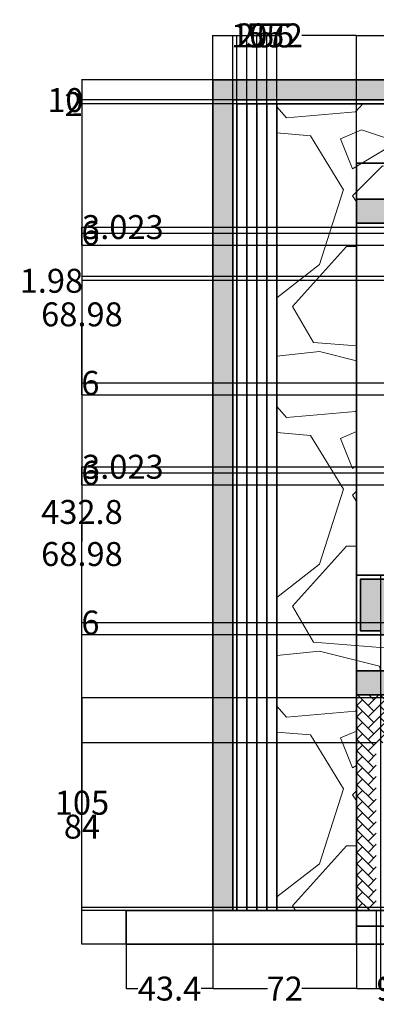
# Model space of a CAD drawing. Units: inches. Extents: x -73 to 458, y -161 to 332.
# Tile 1 of 6: x -73 to 106, y -161 to 332. Entities that reach past the tile are written whole.
import ezdxf

# ---------------------------------------------------------------- set-up
doc = ezdxf.new("R2010")
doc.units = ezdxf.units.IN
doc.header["$MEASUREMENT"] = 0
for name, color, linetype, lineweight in [('A-ANNO-DIMS', 2, 'Continuous', 18), ('A-ELEV', 7, 'Continuous', 35), ('A-ELEV-PATT', 8, 'Continuous', 13)]:
    doc.layers.add(name, color=color, linetype=linetype, lineweight=lineweight)
doc.styles.get("Standard").update_dxf_attribs({"font": 'arial.ttf'})
doc.dimstyles.get("Standard").update_dxf_attribs({"dimtxt": 12, "dimasz": 0.18, "dimexe": 0.18, "dimexo": 0.0625, "dimgap": 0.09, "dimtad": 0, "dimtih": 1, "dimtoh": 1, "dimdec": 0, "dimzin": 0, "dimdsep": 46, "dimlunit": 3, "dimtxsty": 'Standard', "dimcen": 0.09, "dimadec": 0, "dimazin": 0, "dimtfac": 1, "dimtdec": 0, "dimtofl": 0, "dimtmove": 0, "dimatfit": 3, "dimfxl": 1, "dimtolj": 1, "dimtzin": 0, "dimarcsym": 0})

# ---------------------------------------------------------------- blocks, each defined once
blk = doc.blocks.new('*D5')
at = {"layer": 'A-ANNO-DIMS', "color": 0, "lineweight": -2, "transparency": 16777216}
for p, q in [((24, 302.08), (24, 324.4)), ((24.18, 324.22), (51.42, 324.22)), ((95.82, 324.22), (68.57, 324.22)), ((96, 260.27), (96, 324.4))]:
    blk.add_line(p, q, dxfattribs=at)
at = {"layer": 'A-ANNO-DIMS', "color": 0, "transparency": 16777216}
for points in [[(24.18, 324.25), (24.18, 324.19), (24, 324.22)], [(95.82, 324.25), (95.82, 324.19), (96, 324.22)]]:
    blk.add_solid(points, dxfattribs=at)
at = {"layer": 'Defpoints', "color": 0, "transparency": 16777216}
for p in [(96, 324.22), (24, 302.02), (96, 260.21)]:
    blk.add_point(p, dxfattribs=at)
at = {"layer": 'A-ANNO-DIMS', "color": 0, "transparency": 16777216, "insert": (60, 324.22), "char_height": 12, "attachment_point": 5}
blk.add_mtext('\\A1;72', dxfattribs=at)
blk = doc.blocks.new('*D6')
at = {"layer": 'A-ANNO-DIMS', "color": 0, "lineweight": -2, "transparency": 16777216}
for p, q in [((96, 260.27), (96, 324.4)), ((96.18, 324.22), (126.35, 324.22)), ((173.82, 324.22), (143.65, 324.22)), ((174, 126.13), (174, 324.4))]:
    blk.add_line(p, q, dxfattribs=at)
at = {"layer": 'A-ANNO-DIMS', "color": 0, "transparency": 16777216}
for points in [[(96.18, 324.25), (96.18, 324.19), (96, 324.22)], [(173.82, 324.25), (173.82, 324.19), (174, 324.22)]]:
    blk.add_solid(points, dxfattribs=at)
at = {"layer": 'Defpoints', "color": 0, "transparency": 16777216}
for p in [(174, 324.22), (96, 260.21), (174, 126.07)]:
    blk.add_point(p, dxfattribs=at)
at = {"layer": 'A-ANNO-DIMS', "color": 0, "transparency": 16777216, "insert": (135, 324.22), "char_height": 12, "attachment_point": 5}
blk.add_mtext('\\A1;78', dxfattribs=at)
blk = doc.blocks.new('*D9')
at = {"layer": 'A-ANNO-DIMS', "color": 0, "lineweight": -2, "transparency": 16777216}
for p, q in [((24, -114), (24, -153.17)), ((-19.4, -130.85), (-19.4, -153.17)), ((-19.22, -152.99), (-13.59, -152.99)), ((23.82, -152.99), (18.19, -152.99))]:
    blk.add_line(p, q, dxfattribs=at)
at = {"layer": 'A-ANNO-DIMS', "color": 0, "transparency": 16777216}
for points in [[(-19.22, -152.96), (-19.22, -153.02), (-19.4, -152.99)], [(23.82, -152.96), (23.82, -153.02), (24, -152.99)]]:
    blk.add_solid(points, dxfattribs=at)
at = {"layer": 'Defpoints', "color": 0, "transparency": 16777216}
for p in [(24, -113.93), (-19.4, -130.79), (24, -152.99)]:
    blk.add_point(p, dxfattribs=at)
at = {"layer": 'A-ANNO-DIMS', "color": 0, "transparency": 16777216, "insert": (2.3, -152.99), "char_height": 12, "attachment_point": 5}
blk.add_mtext('\\A1;43.4', dxfattribs=at)
blk = doc.blocks.new('*D10')
at = {"layer": 'A-ANNO-DIMS', "color": 0, "lineweight": -2, "transparency": 16777216}
for p, q in [((24, -114), (24, -153.17)), ((96, -114), (96, -153.17)), ((24.18, -152.99), (51.42, -152.99)), ((95.82, -152.99), (68.57, -152.99))]:
    blk.add_line(p, q, dxfattribs=at)
at = {"layer": 'A-ANNO-DIMS', "color": 0, "transparency": 16777216}
for points in [[(24.18, -152.96), (24.18, -153.02), (24, -152.99)], [(95.82, -152.96), (95.82, -153.02), (96, -152.99)]]:
    blk.add_solid(points, dxfattribs=at)
at = {"layer": 'Defpoints', "color": 0, "transparency": 16777216}
for p in [(24, -113.93), (96, -113.93), (96, -152.99)]:
    blk.add_point(p, dxfattribs=at)
at = {"layer": 'A-ANNO-DIMS', "color": 0, "transparency": 16777216, "insert": (60, -152.99), "char_height": 12, "attachment_point": 5}
blk.add_mtext('\\A1;72', dxfattribs=at)
blk = doc.blocks.new('*D11')
at = {"layer": 'A-ANNO-DIMS', "color": 0, "lineweight": -2, "transparency": 16777216}
for p, q in [((96, -114), (96, -153.17)), ((105.91, -113.98), (105.91, -153.17)), ((96.18, -152.99), (105.73, -152.99)), ((105.91, -152.99), (106.09, -152.99))]:
    blk.add_line(p, q, dxfattribs=at)
at = {"layer": 'A-ANNO-DIMS', "color": 0, "transparency": 16777216}
for points in [[(96.18, -152.96), (96.18, -153.02), (96, -152.99)], [(105.73, -152.96), (105.73, -153.02), (105.91, -152.99)]]:
    blk.add_solid(points, dxfattribs=at)
at = {"layer": 'Defpoints', "color": 0, "transparency": 16777216}
for p in [(96, -113.93), (105.91, -113.92), (105.91, -152.99)]:
    blk.add_point(p, dxfattribs=at)
at = {"layer": 'A-ANNO-DIMS', "color": 0, "transparency": 16777216, "insert": (126.43, -152.99), "char_height": 12, "attachment_point": 5}
blk.add_mtext('\\A1;9.917', dxfattribs=at)
blk = doc.blocks.new('*D12')
at = {"layer": 'A-ANNO-DIMS', "color": 0, "lineweight": -2, "transparency": 16777216}
for p, q in [((105.91, -113.98), (105.91, -153.17)), ((145.91, -113.98), (145.91, -153.17)), ((106.09, -152.99), (117.01, -152.99)), ((145.73, -152.99), (134.82, -152.99))]:
    blk.add_line(p, q, dxfattribs=at)
at = {"layer": 'A-ANNO-DIMS', "color": 0, "transparency": 16777216}
for points in [[(106.09, -152.96), (106.09, -153.02), (105.91, -152.99)], [(145.73, -152.96), (145.73, -153.02), (145.91, -152.99)]]:
    blk.add_solid(points, dxfattribs=at)
at = {"layer": 'Defpoints', "color": 0, "transparency": 16777216}
for p in [(105.91, -113.92), (145.91, -113.92), (145.91, -152.99)]:
    blk.add_point(p, dxfattribs=at)
at = {"layer": 'A-ANNO-DIMS', "color": 0, "transparency": 16777216, "insert": (125.91, -152.99), "char_height": 12, "attachment_point": 5}
blk.add_mtext('\\A1;40', dxfattribs=at)
blk = doc.blocks.new('*D26')
at = {"layer": 'A-ANNO-DIMS', "color": 0, "lineweight": -2, "transparency": 16777216}
for p, q in [((23.94, 302.02), (-41.78, 302.02)), ((-41.6, 301.84), (-41.6, 91.84)), ((-41.6, -130.61), (-41.6, 79.4)), ((-19.47, -130.79), (-41.78, -130.79))]:
    blk.add_line(p, q, dxfattribs=at)
at = {"layer": 'A-ANNO-DIMS', "color": 0, "transparency": 16777216}
for points in [[(-41.63, 301.84), (-41.57, 301.84), (-41.6, 302.02)], [(-41.63, -130.61), (-41.57, -130.61), (-41.6, -130.79)]]:
    blk.add_solid(points, dxfattribs=at)
at = {"layer": 'Defpoints', "color": 0, "transparency": 16777216}
for p in [(-41.6, 302.02), (24, 302.02), (-19.4, -130.79)]:
    blk.add_point(p, dxfattribs=at)
at = {"layer": 'A-ANNO-DIMS', "color": 0, "transparency": 16777216, "insert": (-41.6, 85.62), "char_height": 12, "attachment_point": 5}
blk.add_mtext('\\A1;432.8', dxfattribs=at)
blk = doc.blocks.new('*D27')
at = {"layer": 'A-ANNO-DIMS', "color": 0, "lineweight": -2, "transparency": 16777216}
for p, q in [((105.85, -29.92), (-41.78, -29.92)), ((-41.6, -30.1), (-41.6, -65.7)), ((-41.6, -113.74), (-41.6, -78.14)), ((105.85, -113.92), (-41.78, -113.92))]:
    blk.add_line(p, q, dxfattribs=at)
at = {"layer": 'A-ANNO-DIMS', "color": 0, "transparency": 16777216}
for points in [[(-41.63, -30.1), (-41.57, -30.1), (-41.6, -29.92)], [(-41.63, -113.74), (-41.57, -113.74), (-41.6, -113.92)]]:
    blk.add_solid(points, dxfattribs=at)
at = {"layer": 'Defpoints', "color": 0, "transparency": 16777216}
for p in [(-41.6, -29.92), (105.91, -29.92), (105.91, -113.92)]:
    blk.add_point(p, dxfattribs=at)
at = {"layer": 'A-ANNO-DIMS', "color": 0, "transparency": 16777216, "insert": (-41.6, -71.92), "char_height": 12, "attachment_point": 5}
blk.add_mtext('\\A1;84', dxfattribs=at)
blk = doc.blocks.new('*D28')
at = {"layer": 'A-ANNO-DIMS', "color": 0, "lineweight": -2, "transparency": 16777216}
for p, q in [((24, 302.08), (24, 324.4)), ((24.18, 324.22), (33.82, 324.22)), ((34, 292.08), (34, 324.4)), ((34, 324.22), (34.18, 324.22))]:
    blk.add_line(p, q, dxfattribs=at)
at = {"layer": 'A-ANNO-DIMS', "color": 0, "transparency": 16777216}
for points in [[(24.18, 324.25), (24.18, 324.19), (24, 324.22)], [(33.82, 324.25), (33.82, 324.19), (34, 324.22)]]:
    blk.add_solid(points, dxfattribs=at)
at = {"layer": 'Defpoints', "color": 0, "transparency": 16777216}
for p in [(34, 324.22), (24, 302.02), (34, 292.02)]:
    blk.add_point(p, dxfattribs=at)
at = {"layer": 'A-ANNO-DIMS', "color": 0, "transparency": 16777216, "insert": (42.28, 324.22), "char_height": 12, "attachment_point": 5}
blk.add_mtext('\\A1;10', dxfattribs=at)
blk = doc.blocks.new('*D29')
at = {"layer": 'A-ANNO-DIMS', "color": 0, "lineweight": -2, "transparency": 16777216}
for p, q in [((34, 292.08), (34, 324.4)), ((34.18, 324.22), (35.82, 324.22)), ((36, 290.08), (36, 324.4)), ((36, 324.22), (36.18, 324.22))]:
    blk.add_line(p, q, dxfattribs=at)
at = {"layer": 'A-ANNO-DIMS', "color": 0, "transparency": 16777216}
for points in [[(34.18, 324.25), (34.18, 324.19), (34, 324.22)], [(35.82, 324.25), (35.82, 324.19), (36, 324.22)]]:
    blk.add_solid(points, dxfattribs=at)
at = {"layer": 'Defpoints', "color": 0, "transparency": 16777216}
for p in [(36, 324.22), (34, 292.02), (36, 290.02)]:
    blk.add_point(p, dxfattribs=at)
at = {"layer": 'A-ANNO-DIMS', "color": 0, "transparency": 16777216, "insert": (40.24, 324.22), "char_height": 12, "attachment_point": 5}
blk.add_mtext('\\A1;2', dxfattribs=at)
blk = doc.blocks.new('*D30')
at = {"layer": 'A-ANNO-DIMS', "color": 0, "lineweight": -2, "transparency": 16777216}
for p, q in [((36, 290.08), (36, 324.4)), ((36.18, 324.22), (40.82, 324.22)), ((41, 290.08), (41, 324.4)), ((41, 324.22), (41.18, 324.22))]:
    blk.add_line(p, q, dxfattribs=at)
at = {"layer": 'A-ANNO-DIMS', "color": 0, "transparency": 16777216}
for points in [[(36.18, 324.25), (36.18, 324.19), (36, 324.22)], [(40.82, 324.25), (40.82, 324.19), (41, 324.22)]]:
    blk.add_solid(points, dxfattribs=at)
at = {"layer": 'Defpoints', "color": 0, "transparency": 16777216}
for p in [(41, 324.22), (36, 290.02), (41, 290.02)]:
    blk.add_point(p, dxfattribs=at)
at = {"layer": 'A-ANNO-DIMS', "color": 0, "transparency": 16777216, "insert": (45.25, 324.22), "char_height": 12, "attachment_point": 5}
blk.add_mtext('\\A1;5', dxfattribs=at)
blk = doc.blocks.new('*D31')
at = {"layer": 'A-ANNO-DIMS', "color": 0, "lineweight": -2, "transparency": 16777216}
for p, q in [((41, 290.08), (41, 324.4)), ((41.18, 324.22), (45.82, 324.22)), ((46, 290.08), (46, 324.4)), ((46, 324.22), (46.18, 324.22))]:
    blk.add_line(p, q, dxfattribs=at)
at = {"layer": 'A-ANNO-DIMS', "color": 0, "transparency": 16777216}
for points in [[(41.18, 324.25), (41.18, 324.19), (41, 324.22)], [(45.82, 324.25), (45.82, 324.19), (46, 324.22)]]:
    blk.add_solid(points, dxfattribs=at)
at = {"layer": 'Defpoints', "color": 0, "transparency": 16777216}
for p in [(46, 324.22), (41, 290.02), (46, 290.02)]:
    blk.add_point(p, dxfattribs=at)
at = {"layer": 'A-ANNO-DIMS', "color": 0, "transparency": 16777216, "insert": (50.25, 324.22), "char_height": 12, "attachment_point": 5}
blk.add_mtext('\\A1;5', dxfattribs=at)
blk = doc.blocks.new('*D32')
at = {"layer": 'A-ANNO-DIMS', "color": 0, "lineweight": -2, "transparency": 16777216}
for p, q in [((46, 290.08), (46, 324.4)), ((46.18, 324.22), (50.82, 324.22)), ((51, 290.08), (51, 324.4)), ((51, 324.22), (51.18, 324.22))]:
    blk.add_line(p, q, dxfattribs=at)
at = {"layer": 'A-ANNO-DIMS', "color": 0, "transparency": 16777216}
for points in [[(46.18, 324.25), (46.18, 324.19), (46, 324.22)], [(50.82, 324.25), (50.82, 324.19), (51, 324.22)]]:
    blk.add_solid(points, dxfattribs=at)
at = {"layer": 'Defpoints', "color": 0, "transparency": 16777216}
for p in [(51, 324.22), (46, 290.02), (51, 290.02)]:
    blk.add_point(p, dxfattribs=at)
at = {"layer": 'A-ANNO-DIMS', "color": 0, "transparency": 16777216, "insert": (55.25, 324.22), "char_height": 12, "attachment_point": 5}
blk.add_mtext('\\A1;5', dxfattribs=at)
blk = doc.blocks.new('*D33')
at = {"layer": 'A-ANNO-DIMS', "color": 0, "lineweight": -2, "transparency": 16777216}
for p, q in [((51, 290.08), (51, 324.4)), ((51.18, 324.22), (55.82, 324.22)), ((56, 290.08), (56, 324.4)), ((56, 324.22), (56.18, 324.22))]:
    blk.add_line(p, q, dxfattribs=at)
at = {"layer": 'A-ANNO-DIMS', "color": 0, "transparency": 16777216}
for points in [[(51.18, 324.25), (51.18, 324.19), (51, 324.22)], [(55.82, 324.25), (55.82, 324.19), (56, 324.22)]]:
    blk.add_solid(points, dxfattribs=at)
at = {"layer": 'Defpoints', "color": 0, "transparency": 16777216}
for p in [(56, 324.22), (51, 290.02), (56, 290.02)]:
    blk.add_point(p, dxfattribs=at)
at = {"layer": 'A-ANNO-DIMS', "color": 0, "transparency": 16777216, "insert": (60.25, 324.22), "char_height": 12, "attachment_point": 5}
blk.add_mtext('\\A1;5', dxfattribs=at)
blk = doc.blocks.new('*D34')
at = {"layer": 'A-ANNO-DIMS', "color": 0, "lineweight": -2, "transparency": 16777216}
for p, q in [((23.94, 302.02), (-41.78, 302.02)), ((-41.6, 301.84), (-41.6, 292.2)), ((33.94, 292.02), (-41.78, 292.02)), ((-41.6, 291.84), (-41.78, 291.84)), ((-41.6, 292.02), (-41.6, 291.84))]:
    blk.add_line(p, q, dxfattribs=at)
at = {"layer": 'A-ANNO-DIMS', "color": 0, "transparency": 16777216}
for points in [[(-41.63, 301.84), (-41.57, 301.84), (-41.6, 302.02)], [(-41.63, 292.2), (-41.57, 292.2), (-41.6, 292.02)]]:
    blk.add_solid(points, dxfattribs=at)
at = {"layer": 'Defpoints', "color": 0, "transparency": 16777216}
for p in [(24, 302.02), (-41.6, 292.02), (34, 292.02)]:
    blk.add_point(p, dxfattribs=at)
at = {"layer": 'A-ANNO-DIMS', "color": 0, "transparency": 16777216, "insert": (-49.88, 291.84), "char_height": 12, "attachment_point": 5}
blk.add_mtext('\\A1;10', dxfattribs=at)
blk = doc.blocks.new('*D35')
at = {"layer": 'A-ANNO-DIMS', "color": 0, "lineweight": -2, "transparency": 16777216}
for p, q in [((33.94, 292.02), (-41.78, 292.02)), ((-41.6, 291.84), (-41.6, 290.2)), ((35.94, 290.02), (-41.78, 290.02)), ((-41.6, 289.84), (-41.78, 289.84)), ((-41.6, 290.02), (-41.6, 289.84))]:
    blk.add_line(p, q, dxfattribs=at)
at = {"layer": 'A-ANNO-DIMS', "color": 0, "transparency": 16777216}
for points in [[(-41.63, 291.84), (-41.57, 291.84), (-41.6, 292.02)], [(-41.63, 290.2), (-41.57, 290.2), (-41.6, 290.02)]]:
    blk.add_solid(points, dxfattribs=at)
at = {"layer": 'Defpoints', "color": 0, "transparency": 16777216}
for p in [(34, 292.02), (-41.6, 290.02), (36, 290.02)]:
    blk.add_point(p, dxfattribs=at)
at = {"layer": 'A-ANNO-DIMS', "color": 0, "transparency": 16777216, "insert": (-45.85, 289.84), "char_height": 12, "attachment_point": 5}
blk.add_mtext('\\A1;2', dxfattribs=at)
blk = doc.blocks.new('*D36')
at = {"layer": 'A-ANNO-DIMS', "color": 0, "lineweight": -2, "transparency": 16777216}
for p, q in [((96, 53.96), (96, -153.17)), ((108, 53.96), (108, -153.17)), ((96.18, -152.99), (107.82, -152.99)), ((108, -152.99), (108.18, -152.99))]:
    blk.add_line(p, q, dxfattribs=at)
at = {"layer": 'A-ANNO-DIMS', "color": 0, "transparency": 16777216}
for points in [[(96.18, -152.96), (96.18, -153.02), (96, -152.99)], [(107.82, -152.96), (107.82, -153.02), (108, -152.99)]]:
    blk.add_solid(points, dxfattribs=at)
at = {"layer": 'Defpoints', "color": 0, "transparency": 16777216}
for p in [(96, 54.03), (108, 54.03), (108, -152.99)]:
    blk.add_point(p, dxfattribs=at)
at = {"layer": 'A-ANNO-DIMS', "color": 0, "transparency": 16777216, "insert": (116.24, -152.99), "char_height": 12, "attachment_point": 5}
blk.add_mtext('\\A1;12', dxfattribs=at)
blk = doc.blocks.new('*D47')
at = {"layer": 'A-ANNO-DIMS', "color": 0, "lineweight": -2, "transparency": 16777216}
for p, q in [((143.94, 203.54), (-41.78, 203.54)), ((-41.6, 203.36), (-41.6, 201.74)), ((143.94, 201.56), (-41.78, 201.56)), ((-41.6, 201.38), (-41.78, 201.38)), ((-41.6, 201.56), (-41.6, 201.38))]:
    blk.add_line(p, q, dxfattribs=at)
at = {"layer": 'A-ANNO-DIMS', "color": 0, "transparency": 16777216}
for points in [[(-41.63, 203.36), (-41.57, 203.36), (-41.6, 203.54)], [(-41.63, 201.74), (-41.57, 201.74), (-41.6, 201.56)]]:
    blk.add_solid(points, dxfattribs=at)
at = {"layer": 'Defpoints', "color": 0, "transparency": 16777216}
for p in [(144, 203.54), (-41.6, 201.56), (144, 201.56)]:
    blk.add_point(p, dxfattribs=at)
at = {"layer": 'A-ANNO-DIMS', "color": 0, "transparency": 16777216, "insert": (-56.91, 201.38), "char_height": 12, "attachment_point": 5}
blk.add_mtext('\\A1;1.98', dxfattribs=at)
blk = doc.blocks.new('*D61')
at = {"layer": 'A-ANNO-DIMS', "color": 0, "lineweight": -2, "transparency": 16777216}
for p, q in [((241.74, 150.08), (-41.78, 150.08)), ((-41.6, 150.08), (-41.6, 150.26)), ((-41.6, 150.26), (-41.42, 150.26)), ((-41.6, 144.26), (-41.6, 149.9)), ((248.74, 144.08), (-41.78, 144.08))]:
    blk.add_line(p, q, dxfattribs=at)
at = {"layer": 'A-ANNO-DIMS', "color": 0, "transparency": 16777216}
for points in [[(-41.63, 149.9), (-41.57, 149.9), (-41.6, 150.08)], [(-41.63, 144.26), (-41.57, 144.26), (-41.6, 144.08)]]:
    blk.add_solid(points, dxfattribs=at)
at = {"layer": 'Defpoints', "color": 0, "transparency": 16777216}
for p in [(-41.6, 150.08), (241.81, 150.08), (248.81, 144.08)]:
    blk.add_point(p, dxfattribs=at)
at = {"layer": 'A-ANNO-DIMS', "color": 0, "transparency": 16777216, "insert": (-37.37, 150.26), "char_height": 12, "attachment_point": 5}
blk.add_mtext('\\A1;6', dxfattribs=at)
blk = doc.blocks.new('*D62')
at = {"layer": 'A-ANNO-DIMS', "color": 0, "lineweight": -2, "transparency": 16777216}
for p, q in [((241.74, 219.06), (-41.78, 219.06)), ((-41.6, 218.88), (-41.6, 190.78)), ((-41.6, 150.26), (-41.6, 178.35)), ((241.74, 150.08), (-41.78, 150.08))]:
    blk.add_line(p, q, dxfattribs=at)
at = {"layer": 'A-ANNO-DIMS', "color": 0, "transparency": 16777216}
for points in [[(-41.63, 218.88), (-41.57, 218.88), (-41.6, 219.06)], [(-41.63, 150.26), (-41.57, 150.26), (-41.6, 150.08)]]:
    blk.add_solid(points, dxfattribs=at)
at = {"layer": 'Defpoints', "color": 0, "transparency": 16777216}
for p in [(-41.6, 219.06), (241.81, 219.06), (241.81, 150.08)]:
    blk.add_point(p, dxfattribs=at)
at = {"layer": 'A-ANNO-DIMS', "color": 0, "transparency": 16777216, "insert": (-41.6, 184.57), "char_height": 12, "attachment_point": 5}
blk.add_mtext('\\A1;68.98', dxfattribs=at)
blk = doc.blocks.new('*D63')
at = {"layer": 'A-ANNO-DIMS', "color": 0, "lineweight": -2, "transparency": 16777216}
for p, q in [((245.74, 225.06), (-41.78, 225.06)), ((-41.6, 225.06), (-41.6, 225.24)), ((-41.6, 225.24), (-41.42, 225.24)), ((-41.6, 219.24), (-41.6, 224.88)), ((241.74, 219.06), (-41.78, 219.06))]:
    blk.add_line(p, q, dxfattribs=at)
at = {"layer": 'A-ANNO-DIMS', "color": 0, "transparency": 16777216}
for points in [[(-41.63, 224.88), (-41.57, 224.88), (-41.6, 225.06)], [(-41.63, 219.24), (-41.57, 219.24), (-41.6, 219.06)]]:
    blk.add_solid(points, dxfattribs=at)
at = {"layer": 'Defpoints', "color": 0, "transparency": 16777216}
for p in [(-41.6, 225.06), (245.81, 225.06), (241.81, 219.06)]:
    blk.add_point(p, dxfattribs=at)
at = {"layer": 'A-ANNO-DIMS', "color": 0, "transparency": 16777216, "insert": (-37.37, 225.24), "char_height": 12, "attachment_point": 5}
blk.add_mtext('\\A1;6', dxfattribs=at)
blk = doc.blocks.new('*D64')
at = {"layer": 'A-ANNO-DIMS', "color": 0, "lineweight": -2, "transparency": 16777216}
for p, q in [((248.74, 228.08), (-41.78, 228.08)), ((-41.6, 228.08), (-41.6, 228.26)), ((-41.6, 228.26), (-41.42, 228.26)), ((-41.6, 225.24), (-41.6, 227.9)), ((245.74, 225.06), (-41.78, 225.06))]:
    blk.add_line(p, q, dxfattribs=at)
at = {"layer": 'A-ANNO-DIMS', "color": 0, "transparency": 16777216}
for points in [[(-41.63, 227.9), (-41.57, 227.9), (-41.6, 228.08)], [(-41.63, 225.24), (-41.57, 225.24), (-41.6, 225.06)]]:
    blk.add_solid(points, dxfattribs=at)
at = {"layer": 'Defpoints', "color": 0, "transparency": 16777216}
for p in [(-41.6, 228.08), (248.81, 228.08), (245.81, 225.06)]:
    blk.add_point(p, dxfattribs=at)
at = {"layer": 'A-ANNO-DIMS', "color": 0, "transparency": 16777216, "insert": (-21.09, 228.26), "char_height": 12, "attachment_point": 5}
blk.add_mtext('\\A1;3.023', dxfattribs=at)
blk = doc.blocks.new('*D65')
at = {"layer": 'A-ANNO-DIMS', "color": 0, "lineweight": -2, "transparency": 16777216}
for p, q in [((241.74, 30.08), (-41.78, 30.08)), ((-41.6, 30.08), (-41.6, 30.26)), ((-41.6, 30.26), (-41.42, 30.26)), ((-41.6, 24.26), (-41.6, 29.9)), ((248.74, 24.08), (-41.78, 24.08))]:
    blk.add_line(p, q, dxfattribs=at)
at = {"layer": 'A-ANNO-DIMS', "color": 0, "transparency": 16777216}
for points in [[(-41.63, 29.9), (-41.57, 29.9), (-41.6, 30.08)], [(-41.63, 24.26), (-41.57, 24.26), (-41.6, 24.08)]]:
    blk.add_solid(points, dxfattribs=at)
at = {"layer": 'Defpoints', "color": 0, "transparency": 16777216}
for p in [(-41.6, 30.08), (241.81, 30.08), (248.81, 24.08)]:
    blk.add_point(p, dxfattribs=at)
at = {"layer": 'A-ANNO-DIMS', "color": 0, "transparency": 16777216, "insert": (-37.37, 30.26), "char_height": 12, "attachment_point": 5}
blk.add_mtext('\\A1;6', dxfattribs=at)
blk = doc.blocks.new('*D66')
at = {"layer": 'A-ANNO-DIMS', "color": 0, "lineweight": -2, "transparency": 16777216}
for p, q in [((241.74, 99.06), (-41.78, 99.06)), ((-41.6, 98.88), (-41.6, 70.78)), ((-41.6, 30.26), (-41.6, 58.35)), ((241.74, 30.08), (-41.78, 30.08))]:
    blk.add_line(p, q, dxfattribs=at)
at = {"layer": 'A-ANNO-DIMS', "color": 0, "transparency": 16777216}
for points in [[(-41.63, 98.88), (-41.57, 98.88), (-41.6, 99.06)], [(-41.63, 30.26), (-41.57, 30.26), (-41.6, 30.08)]]:
    blk.add_solid(points, dxfattribs=at)
at = {"layer": 'Defpoints', "color": 0, "transparency": 16777216}
for p in [(-41.6, 99.06), (241.81, 99.06), (241.81, 30.08)]:
    blk.add_point(p, dxfattribs=at)
at = {"layer": 'A-ANNO-DIMS', "color": 0, "transparency": 16777216, "insert": (-41.6, 64.57), "char_height": 12, "attachment_point": 5}
blk.add_mtext('\\A1;68.98', dxfattribs=at)
blk = doc.blocks.new('*D67')
at = {"layer": 'A-ANNO-DIMS', "color": 0, "lineweight": -2, "transparency": 16777216}
for p, q in [((245.74, 105.06), (-41.78, 105.06)), ((-41.6, 105.06), (-41.6, 105.24)), ((-41.6, 105.24), (-41.42, 105.24)), ((-41.6, 99.24), (-41.6, 104.88)), ((241.74, 99.06), (-41.78, 99.06))]:
    blk.add_line(p, q, dxfattribs=at)
at = {"layer": 'A-ANNO-DIMS', "color": 0, "transparency": 16777216}
for points in [[(-41.63, 104.88), (-41.57, 104.88), (-41.6, 105.06)], [(-41.63, 99.24), (-41.57, 99.24), (-41.6, 99.06)]]:
    blk.add_solid(points, dxfattribs=at)
at = {"layer": 'Defpoints', "color": 0, "transparency": 16777216}
for p in [(-41.6, 105.06), (245.81, 105.06), (241.81, 99.06)]:
    blk.add_point(p, dxfattribs=at)
at = {"layer": 'A-ANNO-DIMS', "color": 0, "transparency": 16777216, "insert": (-37.37, 105.24), "char_height": 12, "attachment_point": 5}
blk.add_mtext('\\A1;6', dxfattribs=at)
blk = doc.blocks.new('*D68')
at = {"layer": 'A-ANNO-DIMS', "color": 0, "lineweight": -2, "transparency": 16777216}
for p, q in [((248.74, 108.08), (-41.78, 108.08)), ((245.74, 105.06), (-41.78, 105.06)), ((-41.6, 108.08), (-41.6, 108.26)), ((-41.6, 108.26), (-41.42, 108.26)), ((-41.6, 105.24), (-41.6, 107.9))]:
    blk.add_line(p, q, dxfattribs=at)
at = {"layer": 'A-ANNO-DIMS', "color": 0, "transparency": 16777216}
for points in [[(-41.63, 107.9), (-41.57, 107.9), (-41.6, 108.08)], [(-41.63, 105.24), (-41.57, 105.24), (-41.6, 105.06)]]:
    blk.add_solid(points, dxfattribs=at)
at = {"layer": 'Defpoints', "color": 0, "transparency": 16777216}
for p in [(-41.6, 108.08), (245.81, 105.06), (248.81, 108.08)]:
    blk.add_point(p, dxfattribs=at)
at = {"layer": 'A-ANNO-DIMS', "color": 0, "transparency": 16777216, "insert": (-21.09, 108.26), "char_height": 12, "attachment_point": 5}
blk.add_mtext('\\A1;3.023', dxfattribs=at)
blk = doc.blocks.new('*D81')
at = {"layer": 'A-ANNO-DIMS', "color": 0, "lineweight": -2, "transparency": 16777216}
for p, q in [((203.79, -7.43), (-41.78, -7.43)), ((-41.6, -7.61), (-41.6, -53.72)), ((-41.6, -112.25), (-41.6, -66.15)), ((203.79, -112.43), (-41.78, -112.43))]:
    blk.add_line(p, q, dxfattribs=at)
at = {"layer": 'A-ANNO-DIMS', "color": 0, "transparency": 16777216}
for points in [[(-41.63, -7.61), (-41.57, -7.61), (-41.6, -7.43)], [(-41.63, -112.25), (-41.57, -112.25), (-41.6, -112.43)]]:
    blk.add_solid(points, dxfattribs=at)
at = {"layer": 'Defpoints', "color": 0, "transparency": 16777216}
for p in [(-41.6, -7.43), (203.85, -7.43), (203.85, -112.43)]:
    blk.add_point(p, dxfattribs=at)
at = {"layer": 'A-ANNO-DIMS', "color": 0, "transparency": 16777216, "insert": (-41.6, -59.93), "char_height": 12, "attachment_point": 5}
blk.add_mtext('\\A1;105', dxfattribs=at)

msp = doc.modelspace()

# ---------------------------------------------------------------- hatches: boundary and pattern name
at = {"layer": 'A-ELEV-PATT'}
h = msp.add_hatch(color=256, dxfattribs=at)
h.dxf.hatch_style = 1
h.paths.add_polyline_path([(167.9979, 302.0202), (155.9979, 302.0202), (95.9979, 302.0202), (23.9979, 302.0202), (23.9979, -113.9335), (33.9979, -113.9335), (33.9979, 292.0202), (95.9979, 292.0202), (157.9979, 292.0202), (157.9979, 260.2059), (167.9979, 260.2059), (167.9979, 290.0202)])
h.paths.add_polyline_path([(335.9979, 242.2059), (323.9979, 242.2059), (95.9979, 242.2059), (95.9979, 234.0665), (95.9979, 230.2059), (323.9979, 230.2059), (335.9979, 230.2059)])
h.paths.add_polyline_path([(335.9979, 126.0665), (323.9979, 126.0665), (173.9979, 126.0665), (173.9979, 114.0665), (323.9979, 114.0665), (335.9979, 114.0665)])
h.paths.add_polyline_path([(335.9979, 6.0665), (323.9979, 6.0665), (95.9979, 6.0665), (95.9979, -5.9335), (323.9979, -5.9335), (335.9979, -5.9335)])
h = msp.add_hatch(dxfattribs=at)
h.set_pattern_fill('GRAVEL', color=256, scale=150)
h.paths.add_polyline_path([(95.9979, 234.0665), (95.9979, 260.2059), (155.9979, 260.2059), (155.9979, 290.0202), (95.9979, 290.0202), (55.9979, 290.0202), (55.9979, -113.9335), (95.9979, -113.9335), (95.9979, 24.0665), (95.9979, 54.0267)])
h.paths.add_polyline_path([(323.9979, 144.0665), (248.9979, 144.0665), (173.9979, 144.0665), (173.9979, 126.0665), (323.9979, 126.0665)])
h.paths.add_polyline_path([(323.9979, 24.0665), (248.9979, 24.0665), (155.9979, 24.0665), (155.9979, 6.0665), (323.9979, 6.0665)])
h.paths.add_polyline_path([(323.9979, 260.2059), (95.9979, 260.2059), (95.9979, 242.2059), (323.9979, 242.2059)])
h.paths.add_polyline_path([(155.9979, 24.0665), (95.9979, 24.0665), (95.9979, 6.0665), (155.9979, 6.0665)], flags=17)
h = msp.add_hatch(color=256, dxfattribs=at)
h.dxf.hatch_style = 1
h.paths.add_polyline_path([(153.9979, 52.0267), (97.9979, 52.0267), (97.9979, 26.0665), (107.9979, 26.0665), (107.9979, 24.0665), (143.9979, 24.0665), (143.9979, 26.0665), (153.9979, 26.0665)])
h = msp.add_hatch(dxfattribs=at)
h.set_pattern_fill('AR-HBONE', color=256)
h.paths.add_polyline_path([(155.3839, -5.9335), (95.9979, -5.9335), (95.9979, -113.9335), (105.915, -113.9335), (105.915, -29.9207), (145.915, -29.9207), (145.915, -113.9335), (155.3839, -113.9335)])

# ---------------------------------------------------------------- linework, layer by layer
at = {"layer": 'A-ELEV'}
for p, q in [((35.9979, 290.0202), (35.9979, -113.9335)), ((40.9979, 290.0202), (40.9979, -113.9335)), ((45.9979, 290.0202), (45.9979, -113.9335)), ((50.9979, 290.0202), (50.9979, -113.9335)), ((55.9979, 290.0202), (55.9979, -113.9335)), ((323.9979, 260.2059), (95.9979, 260.2059)), ((95.9979, 234.0665), (95.9979, 260.2059)), ((323.9979, 242.2059), (95.9979, 242.2059)), ((95.9979, 234.0665), (95.9979, 6.0665)), ((323.9979, 230.2059), (95.9979, 230.2059)), ((95.9979, 27.9482), (95.9979, 9.9482)), ((95.9979, 24.0665), (143.9979, 24.0665)), ((95.9979, 24.0665), (95.9979, -113.9335)), ((95.9979, 6.0665), (323.9979, 6.0665)), ((95.9979, -5.9335), (323.9979, -5.9335)), ((23.9979, -113.9335), (323.9979, -113.9335))]:
    msp.add_line(p, q, dxfattribs=at)
for points in [[(167.9979, 260.2059), (167.9979, 302.0202), (155.9979, 302.0202), (95.9979, 302.0202), (23.9979, 302.0202), (23.9979, -113.9335)], [(157.9979, 260.2059), (157.9979, 292.0202), (95.9979, 292.0202), (33.9979, 292.0202), (33.9979, -113.9335)], [(155.9979, 260.2059), (155.9979, 290.0202), (95.9979, 290.0202), (35.9979, 290.0202), (35.9979, -113.9335)], [(143.9979, 26.0665), (153.9979, 26.0665), (153.9979, 52.0267), (97.9979, 52.0267), (97.9979, 26.0665), (107.9979, 26.0665)]]:
    msp.add_lwpolyline(points, dxfattribs=at)
for points in [[(95.9979, 24.0665), (155.9979, 24.0665), (155.9979, 54.0267), (95.9979, 54.0267)], [(386.126, -113.9335), (-19.4031, -113.9335), (-19.4031, -130.7857), (386.126, -130.7857)], [(95.9979, -113.9335), (162.3543, -113.9335), (162.3543, -121.6608), (95.9979, -121.6608)], [(95.9979, -121.6608), (162.3543, -121.6608), (162.3543, -130.7857), (95.9979, -130.7857)]]:
    msp.add_lwpolyline(points, close=True, dxfattribs=at)

# ---------------------------------------------------------------- dimensions: what is measured, and where the dimension line sits
at = {"layer": 'A-ANNO-DIMS'}
for base, p1, p2, override, picture, middle in [((95.9979, 324.2202), (23.9979, 302.0202), (95.9979, 260.2059), {"dimdec": 0, "dimlfac": 1, "dimrnd": 0, "dimzin": 0, "dimdsep": 46, "dimlunit": 2}, '*D5', (59.9979, 324.2202)), ((33.9979, 324.2202), (23.9979, 302.0202), (33.9979, 292.0202), {"dimdec": 0, "dimlfac": 1, "dimrnd": 0, "dimzin": 0, "dimdsep": 46, "dimlunit": 2}, '*D28', (42.2774, 324.2202)), ((35.9979, 324.2202), (33.9979, 292.0202), (35.9979, 290.0202), {"dimdec": 0, "dimlfac": 1, "dimrnd": 0, "dimzin": 0, "dimdsep": 46, "dimlunit": 2}, '*D29', (40.2419, 324.2202)), ((40.9979, 324.2202), (35.9979, 290.0202), (40.9979, 290.0202), {"dimdec": 0, "dimlfac": 1, "dimrnd": 0, "dimzin": 0, "dimdsep": 46, "dimlunit": 2}, '*D30', (45.246, 324.2202)), ((45.9979, 324.2202), (40.9979, 290.0202), (45.9979, 290.0202), {"dimdec": 0, "dimlfac": 1, "dimrnd": 0, "dimzin": 0, "dimdsep": 46, "dimlunit": 2}, '*D31', (50.246, 324.2202)), ((50.9979, 324.2202), (45.9979, 290.0202), (50.9979, 290.0202), {"dimdec": 0, "dimlfac": 1, "dimrnd": 0, "dimzin": 0, "dimdsep": 46, "dimlunit": 2}, '*D32', (55.246, 324.2202)), ((55.9979, 324.2202), (50.9979, 290.0202), (55.9979, 290.0202), {"dimdec": 0, "dimlfac": 1, "dimrnd": 0, "dimzin": 0, "dimdsep": 46, "dimlunit": 2}, '*D33', (60.246, 324.2202)), ((173.9979, 324.2202), (95.9979, 260.2059), (173.9979, 126.0665), {"dimdec": 0, "dimlfac": 1, "dimrnd": 0, "dimzin": 0, "dimdsep": 46, "dimlunit": 2}, '*D6', (134.9979, 324.2202)), ((107.9979, -152.9857), (95.9979, 54.0267), (107.9979, 54.0267), {"dimdec": 0, "dimlfac": 1, "dimrnd": 0, "dimzin": 0, "dimdsep": 46, "dimlunit": 2}, '*D36', (116.2365, -152.9857)), ((23.9979, -152.9857), (-19.4031, -130.7857), (23.9979, -113.9335), {"dimdec": 1, "dimlfac": 1, "dimrnd": 0, "dimzin": 0, "dimdsep": 46, "dimlunit": 2}, '*D9', (2.2974, -152.9857)), ((95.9979, -152.9857), (23.9979, -113.9335), (95.9979, -113.9335), {"dimdec": 0, "dimlfac": 1, "dimrnd": 0, "dimzin": 0, "dimdsep": 46, "dimlunit": 2}, '*D10', (59.9979, -152.9857)), ((105.915, -152.9857), (95.9979, -113.9335), (105.915, -113.9207), {"dimdec": 3, "dimlfac": 1, "dimrnd": 0, "dimzin": 0, "dimdsep": 46, "dimlunit": 2}, '*D11', (126.4319, -152.9857)), ((145.915, -152.9857), (105.915, -113.9207), (145.915, -113.9207), {"dimdec": 0, "dimlfac": 1, "dimrnd": 0, "dimzin": 0, "dimdsep": 46, "dimlunit": 2}, '*D12', (125.915, -152.9857))]:
    dim = msp.add_linear_dim(base=base, p1=p1, p2=p2, dimstyle='Standard', override=override, dxfattribs=at)
    dim.commit()
    dim.dimension.update_dxf_attribs({"geometry": picture, "text_midpoint": middle})
for base, p1, p2, override, picture, middle in [((-41.6031, 302.0202), (-19.4031, -130.7857), (23.9979, 302.0202), {"dimdec": 1, "dimlfac": 1, "dimrnd": 0, "dimzin": 0, "dimdsep": 46, "dimlunit": 2}, '*D26', (-41.6031, 85.6173)), ((-41.6031, 292.0202), (23.9979, 302.0202), (33.9979, 292.0202), {"dimdec": 0, "dimlfac": 1, "dimrnd": 0, "dimzin": 0, "dimdsep": 46, "dimlunit": 2}, '*D34', (-49.8827, 291.8402)), ((-41.6031, 290.0202), (33.9979, 292.0202), (35.9979, 290.0202), {"dimdec": 0, "dimlfac": 1, "dimrnd": 0, "dimzin": 0, "dimdsep": 46, "dimlunit": 2}, '*D35', (-45.8472, 289.8402)), ((-41.6031, 225.0563), (241.805, 219.0563), (245.805, 225.0563), {"dimdec": 0, "dimlfac": 1, "dimrnd": 0, "dimzin": 0, "dimdsep": 46, "dimlunit": 2}, '*D63', (-37.3713, 225.2363)), ((-41.6031, 228.0793), (245.805, 225.0563), (248.805, 228.0793), {"dimdec": 3, "dimlfac": 1, "dimrnd": 0, "dimzin": 0, "dimdsep": 46, "dimlunit": 2}, '*D64', (-21.0903, 228.2593)), ((-41.6031, 219.0563), (241.805, 150.0793), (241.805, 219.0563), {"dimdec": 2, "dimlfac": 1, "dimrnd": 0, "dimzin": 0, "dimdsep": 46, "dimlunit": 2}, '*D62', (-41.6031, 184.5678)), ((-41.6031, 201.5578), (143.9979, 203.5354), (143.9979, 201.5578), {"dimdec": 2, "dimlfac": 1, "dimrnd": 0, "dimzin": 0, "dimdsep": 46, "dimlunit": 2}, '*D47', (-56.9059, 201.3778)), ((-41.6031, 150.0793), (248.805, 144.0793), (241.805, 150.0793), {"dimdec": 0, "dimlfac": 1, "dimrnd": 0, "dimzin": 0, "dimdsep": 46, "dimlunit": 2}, '*D61', (-37.3713, 150.2593)), ((-41.6031, 108.0793), (245.805, 105.0563), (248.805, 108.0793), {"dimdec": 3, "dimlfac": 1, "dimrnd": 0, "dimzin": 0, "dimdsep": 46, "dimlunit": 2}, '*D68', (-21.0903, 108.2593)), ((-41.6031, 105.0563), (241.805, 99.0563), (245.805, 105.0563), {"dimdec": 0, "dimlfac": 1, "dimrnd": 0, "dimzin": 0, "dimdsep": 46, "dimlunit": 2}, '*D67', (-37.3713, 105.2363)), ((-41.6031, 99.0563), (241.805, 30.0793), (241.805, 99.0563), {"dimdec": 2, "dimlfac": 1, "dimrnd": 0, "dimzin": 0, "dimdsep": 46, "dimlunit": 2}, '*D66', (-41.6031, 64.5678)), ((-41.6031, 30.0793), (248.805, 24.0793), (241.805, 30.0793), {"dimdec": 0, "dimlfac": 1, "dimrnd": 0, "dimzin": 0, "dimdsep": 46, "dimlunit": 2}, '*D65', (-37.3713, 30.2593)), ((-41.6031, -7.4335), (203.8513, -112.4335), (203.8513, -7.4335), {"dimdec": 0, "dimlfac": 1, "dimrnd": 0, "dimzin": 0, "dimdsep": 46, "dimlunit": 2}, '*D81', (-41.6031, -59.9335)), ((-41.6031, -29.9207), (105.915, -113.9207), (105.915, -29.9207), {"dimdec": 0, "dimlfac": 1, "dimrnd": 0, "dimzin": 0, "dimdsep": 46, "dimlunit": 2}, '*D27', (-41.6031, -71.9207))]:
    dim = msp.add_linear_dim(base=base, p1=p1, p2=p2, angle=90, dimstyle='Standard', override=override, dxfattribs=at)
    dim.commit()
    dim.dimension.update_dxf_attribs({"geometry": picture, "text_midpoint": middle})

doc.saveas('drawing.dxf')
